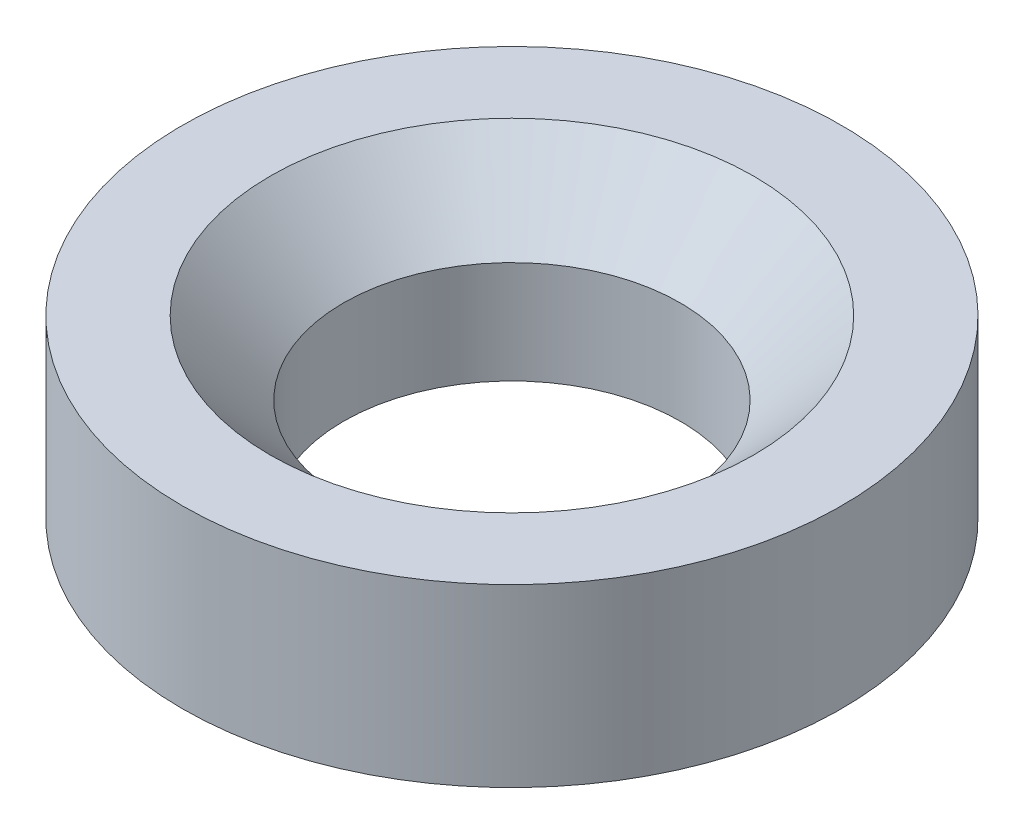
from build123d import *

# Parameters (mm, degrees)
BUSH_OD_PROFILE_45_R  = 22.5
BUSH_BODY_45X12_DEPTH = 12


with BuildPart() as part:
    # Bush OD Profile Ø45 → Bush Body Ø45x12 (new body)
    with BuildSketch(Plane(origin=(0, 0, 0), x_dir=(1, 0, 0), z_dir=(0, 1, 0))):
        with Locations(Location((0, 0, 0), (0, 0, 270))):
            Circle(BUSH_OD_PROFILE_45_R)
    extrude(amount=BUSH_BODY_45X12_DEPTH)

    # Countersunk Bore Profile → Countersunk Bore (revolve, cut)
    with BuildSketch(Plane.XY, mode=Mode.PRIVATE) as countersunk_bore_sk:
        Polygon((11.5, 0), (11.5, 7), (16.5, 12), (0, 12), (0, 0), align=None)
    revolve(countersunk_bore_sk.sketch.rotate(Axis((0, 12, 0), (0, -1, 0)), 180), axis=Axis((0, 12, 0), (0, -1, 0)), mode=Mode.SUBTRACT)


solid = part.part
